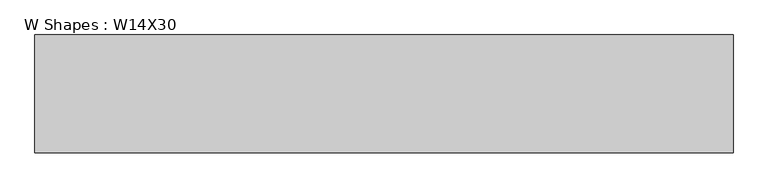
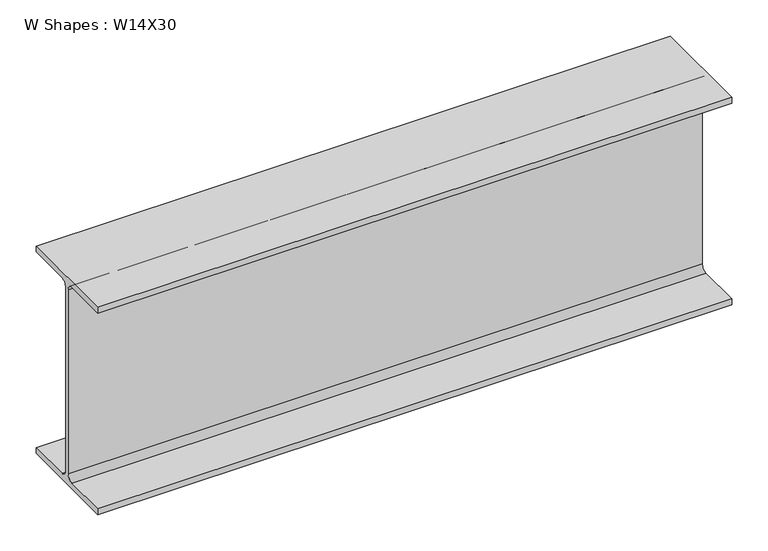
"""IFC4 building model written with IfcOpenShell, lengths in millimetres: beam geometry, W Shapes : W14X30."""

from ifc_helpers import new_model, si_unit, point, frame, frame_2d, origin, place, context, project, spatial, polyline, circle_curve, trimmed, segment, composite_curve, outline, extrude, source, transform, mapped, element, save


def w_shapes_w14x30_95bb247d(model_context):
    return source(origin(), model_context, "Body", "SweptSolid", [
        extrude(outline(composite_curve([segment(polyline([(85.471, -165.481), (85.471, -175.26), (-85.471, -175.26), (-85.471, -165.481), (-13.589, -165.481)]), True, "CONTINUOUS"), segment(trimmed(circle_curve(frame_2d((-13.589, -155.321)), 10.16), [point((-13.589, -165.481))], [point((-3.429, -155.321))], True, "CARTESIAN"), True, "CONTINUOUS"), segment(polyline([(-3.429, -155.321), (-3.429, 155.321)]), True, "CONTINUOUS"), segment(trimmed(circle_curve(frame_2d((-13.589, 155.321)), 10.16), [point((-3.429, 155.321))], [point((-13.589, 165.481))], True, "CARTESIAN"), True, "CONTINUOUS"), segment(polyline([(-13.589, 165.481), (-85.471, 165.481), (-85.471, 175.26), (85.471, 175.26), (85.471, 165.481), (13.589, 165.481)]), True, "CONTINUOUS"), segment(trimmed(circle_curve(frame_2d((13.589, 155.321)), 10.16), [point((13.589, 165.481))], [point((3.429, 155.321))], True, "CARTESIAN"), True, "CONTINUOUS"), segment(polyline([(3.429, 155.321), (3.429, -155.321)]), True, "CONTINUOUS"), segment(trimmed(circle_curve(frame_2d((13.589, -155.321)), 10.16), [point((3.429, -155.321))], [point((13.589, -165.481))], True, "CARTESIAN"), True, "CONTINUOUS"), segment(polyline([(13.589, -165.481), (85.471, -165.481)]), True, "CONTINUOUS")], self_intersect=False)), frame((-137.0216519, 0.0, 0.0), z_axis=(1.0, 0.0, 0.0), x_axis=(0.0, 1.0, 0.0)), (0.0, 0.0, 1.0), 1013.8524887),
    ])


if __name__ == "__main__":
    model = new_model("IFC4")
    model_context = context("Model", 3, world=origin())
    ifc_project = project(units=[si_unit("LENGTHUNIT", "METRE", prefix="MILLI")], contexts=[model_context])
    site = spatial("IfcSite", under=ifc_project)
    building = spatial("IfcBuilding", under=site)
    placement = place(None, origin())
    w_shapes_w14x30_shape = w_shapes_w14x30_95bb247d(model_context)
    element("IfcBeam", 1, ObjectType="W Shapes : W14X30", at=placement, inside=building, context=model_context, shape_type="MappedRepresentation", body=[
        mapped(w_shapes_w14x30_shape, transform((0.0, 0.0, 0.0), x_axis=(1.0, 0.0, 0.0), y_axis=(0.0, 1.0, 0.0), z_axis=(0.0, 0.0, 1.0))),
    ])
    save(model, "model.ifc")

# Revit data of these elements
# Type "W Shapes : W14X30"
#   Section Name Key = "W14X30"
#   Width = 6.730"
#   Web Thickness = 0.270"
#   Web Fillet = 0.400"
#   Warping Constant = 887.00 in⁶
#   Torsional Moment of Inertia = 0.38 in⁴
#   Section Area = 8.85 in²
#   Plastic Modulus weak axis = 8.99 in³
#   Plastic Modulus strong axis = 47.30 in³
#   Perimeter = 4.441 ft²/ft
#   Nominal Weight = 30.00 lbf/ft
#   Moment of Inertia weak axis = 19.60 in⁴
#   Moment of Inertia strong axis = 291.00 in⁴
#   Height = 13.800"
#   Flange Thickness = 0.385"
#   Elastic Modulus weak axis = 5.82 in³
#   Elastic Modulus strong axis = 42.00 in³
#   Clear Web Height = 0' - 11 5/8"
#   Centroid Vertical = 6.900"
#   Centroid Horizontal = 3.365"
#   Bolt Spacing = 0' - 3 1/2"
#   Length [instance default] = 1524 mm
#   Structural Material [instance default] = Steel ASTM A992
#   Principal Axes Angle = 0
# Element 1 (IfcBeam, "W Shapes : W14X30")
#   Length = 3216.562 mm
#   Materials on its faces: "Steel ASTM A992"
# Materials
#   "Steel ASTM A992": class "Metal", colour RGB 199 199 199, transparency 0, Description = "Structural steel 50ksi", Cost = 0
